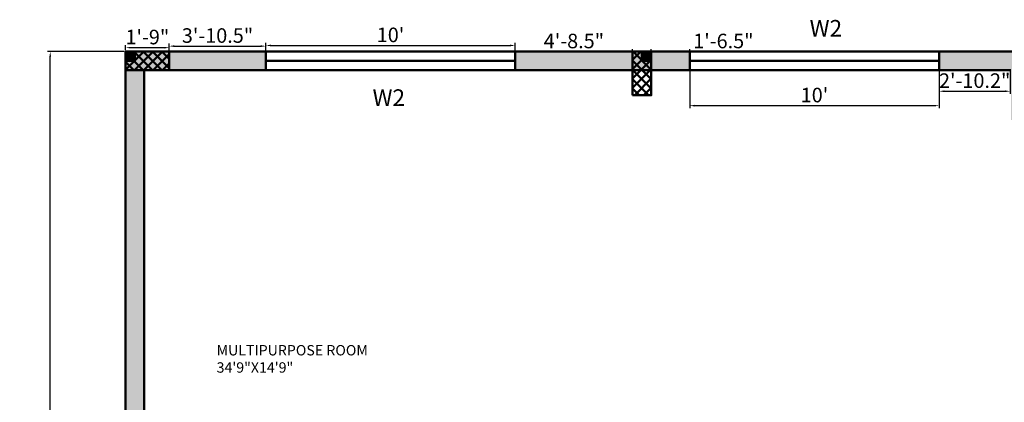
# Model space of a CAD drawing. Units: inches. Extents: x 1749 to 3550, y 1117 to 2383.
# Tile 11 of 15: x 2680 to 3154, y 1503 to 1687. Entities that reach past the tile are written whole.
import ezdxf

# ---------------------------------------------------------------- set-up
doc = ezdxf.new("R2010")
doc.units = ezdxf.units.IN
for name, color, linetype, lineweight in [('A-ANNO-DIMS', 2, 'Continuous', 18), ('A-ANNO-TEXT', 3, 'Continuous', 18), ('A-AREA-IDEN', 7, 'Continuous', 18), ('A-COLS', 10, 'Continuous', 50), ('A-WALL', 7, 'Continuous', 50), ('A-WALL-PATT', 8, 'Continuous', 13)]:
    doc.layers.add(name, color=color, linetype=linetype, lineweight=lineweight)
doc.styles.get("Standard").update_dxf_attribs({"font": 'arial.ttf'})
doc.dimstyles.new('ISO-25', dxfattribs={"dimtxt": 7, "dimasz": 2.5, "dimexe": 1.25, "dimexo": 0.625, "dimtad": 1, "dimdec": 1, "dimlunit": 3, "dimtxsty": 'Standard', "dimcen": 2.5, "dimadec": 0, "dimazin": 0, "dimtfac": 1, "dimtdec": 1, "dimtmove": 0, "dimatfit": 3, "dimfxl": 1, "dimarcsym": 0})

# ---------------------------------------------------------------- blocks, each defined once
blk = doc.blocks.new('*D100')
at = {"layer": 'A-ANNO-DIMS', "color": 0, "lineweight": -2, "ltscale": 0.5, "transparency": 16777216}
for p, q in [((2730.84, 1672.01), (2730.84, 1674.54)), ((2733.34, 1673.29), (2749.34, 1673.29)), ((2751.84, 1672.01), (2751.84, 1674.54))]:
    blk.add_line(p, q, dxfattribs=at)
at = {"layer": 'A-ANNO-DIMS', "color": 0, "ltscale": 0.5, "transparency": 16777216}
for points in [[(2733.34, 1673.7), (2733.34, 1672.87), (2730.84, 1673.29)], [(2749.34, 1673.7), (2749.34, 1672.87), (2751.84, 1673.29)]]:
    blk.add_solid(points, dxfattribs=at)
at = {"layer": 'Defpoints', "color": 0, "ltscale": 0.5, "transparency": 16777216}
for p in [(2751.84, 1673.29), (2730.84, 1671.39), (2751.84, 1671.39)]:
    blk.add_point(p, dxfattribs=at)
at = {"layer": 'A-ANNO-DIMS', "color": 0, "ltscale": 0.5, "transparency": 16777216, "insert": (2741.34, 1677.49), "char_height": 7, "attachment_point": 5}
blk.add_mtext('1\'-9"', dxfattribs=at)
blk = doc.blocks.new('*D101')
at = {"layer": 'A-ANNO-DIMS', "color": 0, "lineweight": -2, "ltscale": 0.5, "transparency": 16777216}
for p, q in [((2751.84, 1672.01), (2751.84, 1675.27)), ((2754.34, 1674.02), (2795.84, 1674.02)), ((2798.34, 1672.01), (2798.34, 1675.27))]:
    blk.add_line(p, q, dxfattribs=at)
at = {"layer": 'A-ANNO-DIMS', "color": 0, "ltscale": 0.5, "transparency": 16777216}
for points in [[(2754.34, 1674.44), (2754.34, 1673.61), (2751.84, 1674.02)], [(2795.84, 1674.44), (2795.84, 1673.61), (2798.34, 1674.02)]]:
    blk.add_solid(points, dxfattribs=at)
at = {"layer": 'Defpoints', "color": 0, "ltscale": 0.5, "transparency": 16777216}
for p in [(2798.34, 1674.02), (2751.84, 1671.39), (2798.34, 1671.39)]:
    blk.add_point(p, dxfattribs=at)
at = {"layer": 'A-ANNO-DIMS', "color": 0, "ltscale": 0.5, "transparency": 16777216, "insert": (2775.09, 1678.22), "char_height": 7, "attachment_point": 5}
blk.add_mtext('3\'-10.5"', dxfattribs=at)
blk = doc.blocks.new('*D102')
at = {"layer": 'A-ANNO-DIMS', "color": 0, "lineweight": -2, "ltscale": 0.5, "transparency": 16777216}
for p, q in [((2798.34, 1672.01), (2798.34, 1675.58)), ((2800.84, 1674.33), (2915.84, 1674.33)), ((2918.34, 1672.01), (2918.34, 1675.58))]:
    blk.add_line(p, q, dxfattribs=at)
at = {"layer": 'A-ANNO-DIMS', "color": 0, "ltscale": 0.5, "transparency": 16777216}
for points in [[(2800.84, 1674.75), (2800.84, 1673.92), (2798.34, 1674.33)], [(2915.84, 1674.75), (2915.84, 1673.92), (2918.34, 1674.33)]]:
    blk.add_solid(points, dxfattribs=at)
at = {"layer": 'Defpoints', "color": 0, "ltscale": 0.5, "transparency": 16777216}
for p in [(2918.34, 1674.33), (2798.34, 1671.39), (2918.34, 1671.39)]:
    blk.add_point(p, dxfattribs=at)
at = {"layer": 'A-ANNO-DIMS', "color": 0, "ltscale": 0.5, "transparency": 16777216, "insert": (2858.34, 1678.53), "char_height": 7, "attachment_point": 5}
blk.add_mtext("10'", dxfattribs=at)
blk = doc.blocks.new('*D103')
at = {"layer": 'A-ANNO-DIMS', "color": 0, "lineweight": -2, "ltscale": 0.5, "transparency": 16777216}
for p, q in [((2918.34, 1672.01), (2918.34, 1672.64)), ((2974.84, 1672.01), (2974.84, 1672.64)), ((2920.84, 1671.39), (2972.34, 1671.39))]:
    blk.add_line(p, q, dxfattribs=at)
at = {"layer": 'A-ANNO-DIMS', "color": 0, "ltscale": 0.5, "transparency": 16777216}
for points in [[(2920.84, 1671.8), (2920.84, 1670.97), (2918.34, 1671.39)], [(2972.34, 1671.8), (2972.34, 1670.97), (2974.84, 1671.39)]]:
    blk.add_solid(points, dxfattribs=at)
at = {"layer": 'Defpoints', "color": 0, "ltscale": 0.5, "transparency": 16777216}
for p in [(2918.34, 1671.39), (2974.84, 1671.39), (2974.84, 1671.39)]:
    blk.add_point(p, dxfattribs=at)
at = {"layer": 'A-ANNO-DIMS', "color": 0, "ltscale": 0.5, "transparency": 16777216, "insert": (2946.59, 1675.59), "char_height": 7, "attachment_point": 5}
blk.add_mtext('4\'-8.5"', dxfattribs=at)
blk = doc.blocks.new('*D104')
at = {"layer": 'A-ANNO-DIMS', "color": 0, "lineweight": -2, "ltscale": 0.5, "transparency": 16777216}
for p, q in [((2983.84, 1672.01), (2983.84, 1672.64)), ((3002.34, 1672.01), (3002.34, 1672.64)), ((2986.34, 1671.39), (2999.84, 1671.39)), ((3002.34, 1671.39), (3032.19, 1671.39))]:
    blk.add_line(p, q, dxfattribs=at)
at = {"layer": 'A-ANNO-DIMS', "color": 0, "ltscale": 0.5, "transparency": 16777216}
for points in [[(2986.34, 1671.8), (2986.34, 1670.97), (2983.84, 1671.39)], [(2999.84, 1671.8), (2999.84, 1670.97), (3002.34, 1671.39)]]:
    blk.add_solid(points, dxfattribs=at)
at = {"layer": 'Defpoints', "color": 0, "ltscale": 0.5, "transparency": 16777216}
for p in [(2983.84, 1671.39), (3002.34, 1671.39), (3002.34, 1671.39)]:
    blk.add_point(p, dxfattribs=at)
at = {"layer": 'A-ANNO-DIMS', "color": 0, "ltscale": 0.5, "transparency": 16777216, "insert": (3018.51, 1675.59), "char_height": 7, "attachment_point": 5}
blk.add_mtext('1\'-6.5"', dxfattribs=at)
blk = doc.blocks.new('*D105')
at = {"layer": 'A-ANNO-DIMS', "color": 0, "lineweight": -2, "ltscale": 0.5, "transparency": 16777216}
for p, q in [((3002.34, 1661.76), (3002.34, 1644.12)), ((3122.34, 1661.76), (3122.34, 1644.12)), ((3004.84, 1645.37), (3119.84, 1645.37))]:
    blk.add_line(p, q, dxfattribs=at)
at = {"layer": 'A-ANNO-DIMS', "color": 0, "ltscale": 0.5, "transparency": 16777216}
for points in [[(3004.84, 1645.78), (3004.84, 1644.95), (3002.34, 1645.37)], [(3119.84, 1645.78), (3119.84, 1644.95), (3122.34, 1645.37)]]:
    blk.add_solid(points, dxfattribs=at)
at = {"layer": 'Defpoints', "color": 0, "ltscale": 0.5, "transparency": 16777216}
for p in [(3002.34, 1662.39), (3122.34, 1662.39), (3122.34, 1645.37)]:
    blk.add_point(p, dxfattribs=at)
at = {"layer": 'A-ANNO-DIMS', "color": 0, "ltscale": 0.5, "transparency": 16777216, "insert": (3062.34, 1649.57), "char_height": 7, "attachment_point": 5}
blk.add_mtext("10'", dxfattribs=at)
blk = doc.blocks.new('*D106')
at = {"layer": 'A-ANNO-DIMS', "color": 0, "lineweight": -2, "ltscale": 0.5, "transparency": 16777216}
for p, q in [((3122.34, 1661.76), (3122.34, 1651.06)), ((3156.55, 1661.76), (3156.55, 1651.06)), ((3124.84, 1652.31), (3154.05, 1652.31))]:
    blk.add_line(p, q, dxfattribs=at)
at = {"layer": 'A-ANNO-DIMS', "color": 0, "ltscale": 0.5, "transparency": 16777216}
for points in [[(3124.84, 1652.72), (3124.84, 1651.89), (3122.34, 1652.31)], [(3154.05, 1652.72), (3154.05, 1651.89), (3156.55, 1652.31)]]:
    blk.add_solid(points, dxfattribs=at)
at = {"layer": 'Defpoints', "color": 0, "ltscale": 0.5, "transparency": 16777216}
for p in [(3122.34, 1662.39), (3156.55, 1662.39), (3156.55, 1652.31)]:
    blk.add_point(p, dxfattribs=at)
at = {"layer": 'A-ANNO-DIMS', "color": 0, "ltscale": 0.5, "transparency": 16777216, "insert": (3139.44, 1656.51), "char_height": 7, "attachment_point": 5}
blk.add_mtext('2\'-10.2"', dxfattribs=at)
blk = doc.blocks.new('*D200')
at = {"layer": 'A-ANNO-DIMS', "color": 0, "lineweight": -2, "ltscale": 0.5, "transparency": 16777216}
for p, q in [((2730.21, 1671.39), (2693.34, 1671.39)), ((2694.59, 1245.39), (2694.59, 1668.89)), ((2730.21, 1242.89), (2693.34, 1242.89))]:
    blk.add_line(p, q, dxfattribs=at)
at = {"layer": 'A-ANNO-DIMS', "color": 0, "ltscale": 0.5, "transparency": 16777216}
for points in [[(2694.17, 1668.89), (2695, 1668.89), (2694.59, 1671.39)], [(2694.17, 1245.39), (2695, 1245.39), (2694.59, 1242.89)]]:
    blk.add_solid(points, dxfattribs=at)
at = {"layer": 'Defpoints', "color": 0, "ltscale": 0.5, "transparency": 16777216}
for p in [(2694.59, 1671.39), (2730.84, 1671.39), (2730.84, 1242.89)]:
    blk.add_point(p, dxfattribs=at)
at = {"layer": 'A-ANNO-DIMS', "color": 0, "ltscale": 0.5, "transparency": 16777216, "insert": (2690.34, 1457.14), "char_height": 7, "attachment_point": 5, "rotation": 90}
blk.add_mtext('35\'-8 1/2"', dxfattribs=at)

msp = doc.modelspace()

# ---------------------------------------------------------------- hatches: boundary and pattern name
at = {"layer": 'A-COLS', "ltscale": 10}
h = msp.add_hatch(color=256, dxfattribs=at)
h.dxf.hatch_style = 1
h.paths.add_polyline_path([(2730.84, 1666.89), (2735.34, 1666.89), (2735.34, 1671.39), (2730.84, 1671.39)])
h = msp.add_hatch(dxfattribs=at)
h.set_pattern_fill('ANSI37', color=256, angle=180)
h.set_pattern_definition([(225, (4403.08, 3029.4936), (2.245064, -2.245064), []), (315, (4403.08, 3029.4936), (2.245064, 2.245064), [])])
h.paths.add_polyline_path([(2730.84, 1671.39), (2730.84, 1662.39), (2751.84, 1662.39), (2751.84, 1671.39)])
h = msp.add_hatch(dxfattribs=at)
h.set_pattern_fill('ANSI37', color=256, angle=90)
h.set_pattern_definition([(135, (4341.9415, -0.8568), (-2.245064, -2.245064), []), (225, (4341.9415, -0.8568), (2.245064, -2.245064), [])])
h.paths.add_polyline_path([(2983.84, 1671.39), (2974.84, 1671.39), (2974.84, 1650.39), (2983.84, 1650.39)])
h = msp.add_hatch(color=256, dxfattribs=at)
h.dxf.hatch_style = 1
h.paths.add_polyline_path([(2979.34, 1671.39), (2979.34, 1666.89), (2983.84, 1666.89), (2983.84, 1671.39)])
at = {"layer": 'A-WALL-PATT', "ltscale": 0.5}
h = msp.add_hatch(color=256, dxfattribs=at)
h.dxf.hatch_style = 1
h.paths.add_polyline_path([(2798.34, 1662.39), (2798.34, 1671.39), (2730.84, 1671.39), (2730.84, 1464.39), (2739.84, 1464.39), (2739.84, 1476.39), (2847.84, 1476.39), (2847.84, 1444.89), (2851.84, 1444.89), (2851.84, 1481.39), (2905.84, 1481.39), (2905.84, 1411.89), (2887.84, 1411.89), (2887.84, 1407.39), (2905.84, 1407.39), (2905.84, 1395.39), (2909.84, 1395.39), (2909.84, 1407.39), (2973.84, 1407.39), (2983.84, 1407.39), (2983.84, 1425.39), (2974.84, 1425.39), (2974.84, 1416.39), (2914.84, 1416.39), (2914.84, 1476.39), (2974.84, 1476.39), (2974.84, 1467.39), (2983.84, 1467.39), (2983.84, 1476.39), (2983.84, 1485.39), (2739.84, 1485.39), (2739.84, 1662.39)])
h = msp.add_hatch(color=256, dxfattribs=at)
h.dxf.hatch_style = 1
h.paths.add_polyline_path([(2918.34, 1671.39), (2918.34, 1662.39), (3002.34, 1662.39), (3002.34, 1671.39)])
h = msp.add_hatch(color=256, dxfattribs=at)
h.dxf.hatch_style = 1
h.paths.add_polyline_path([(3156.84, 1662.39), (3156.84, 1638.39), (3165.84, 1638.39), (3165.84, 1662.39), (3165.84, 1671.39), (3122.34, 1671.39), (3122.34, 1662.39)])

# ---------------------------------------------------------------- linework, layer by layer
at = {"layer": 'A-COLS', "ltscale": 10}
for points in [[(2730.84, 1666.89), (2730.84, 1671.39), (2735.34, 1671.39), (2735.34, 1666.89)], [(2751.84, 1662.39), (2730.84, 1662.39), (2730.84, 1671.39), (2751.84, 1671.39)], [(2974.84, 1650.39), (2974.84, 1671.39), (2983.84, 1671.39), (2983.84, 1650.39)], [(2979.34, 1671.39), (2983.84, 1671.39), (2983.84, 1666.89), (2979.34, 1666.89)]]:
    msp.add_lwpolyline(points, close=True, dxfattribs=at)
at = {"layer": 'A-WALL', "ltscale": 0.5}
for p, q in [((2730.84, 1671.39), (3390.84, 1671.39)), ((2730.84, 1671.39), (2730.84, 1242.89)), ((2798.34, 1662.39), (2798.34, 1671.39)), ((2918.34, 1662.39), (2918.34, 1671.39)), ((3002.34, 1662.39), (3002.34, 1671.39)), ((3122.34, 1662.39), (3122.34, 1671.39)), ((2798.34, 1666.89), (2918.34, 1666.89)), ((3002.34, 1666.89), (3122.34, 1666.89)), ((2739.84, 1662.39), (3156.84, 1662.39)), ((2739.84, 1662.39), (2739.84, 1485.39))]:
    msp.add_line(p, q, dxfattribs=at)

# ---------------------------------------------------------------- texts
at = {"layer": 'A-ANNO-TEXT', "ltscale": 0.5}
for p in [(3060.02, 1678.61), (2849.7, 1645.23)]:
    msp.add_text('W2', height=8, dxfattribs=at).set_placement(p)
at = {"layer": 'A-AREA-IDEN', "ltscale": 0.5}
for s, p in [('MULTIPURPOSE ROOM', (2774.65, 1525.13)), ('34\'9"X14\'9"', (2774.65, 1516.83))]:
    msp.add_text(s, height=5, dxfattribs=at).set_placement(p)

# ---------------------------------------------------------------- dimensions: what is measured, and where the dimension line sits
at = {"layer": 'A-ANNO-DIMS', "ltscale": 0.5}
for base, p1, p2, picture, middle in [((2751.84, 1673.29), (2730.84, 1671.39), (2751.84, 1671.39), '*D100', (2741.34, 1677.49)), ((2798.34, 1674.02), (2751.84, 1671.39), (2798.34, 1671.39), '*D101', (2775.09, 1678.22)), ((2918.34, 1674.33), (2798.34, 1671.39), (2918.34, 1671.39), '*D102', (2858.34, 1678.53)), ((2974.84, 1671.39), (2918.34, 1671.39), (2974.84, 1671.39), '*D103', (2946.59, 1675.59)), ((3002.34, 1671.39), (2983.84, 1671.39), (3002.34, 1671.39), '*D104', (3018.51, 1675.59)), ((3122.34, 1645.37), (3002.34, 1662.39), (3122.34, 1662.39), '*D105', (3062.34, 1649.57)), ((3156.55, 1652.31), (3122.34, 1662.39), (3156.55, 1662.39), '*D106', (3139.44, 1656.51))]:
    dim = msp.add_linear_dim(base=base, p1=p1, p2=p2, dimstyle='ISO-25', override={"dimclrd": 0, "dimclre": 0, "dimclrt": 0}, dxfattribs=at)
    dim.commit()
    dim.dimension.update_dxf_attribs({"geometry": picture, "text_midpoint": middle})
dim = msp.add_linear_dim(base=(2694.59, 1671.39), p1=(2730.84, 1242.89), p2=(2730.84, 1671.39), angle=90, dimstyle='ISO-25', override={"dimdec": 1, "dimlfac": 1, "dimrnd": 0, "dimzin": 1, "dimdsep": 46, "dimlunit": 4, "dimfrac": 2}, dxfattribs=at)
dim.commit()
dim.dimension.update_dxf_attribs({"geometry": '*D200', "text_midpoint": (2690.34, 1457.14)})

doc.saveas('drawing.dxf')
